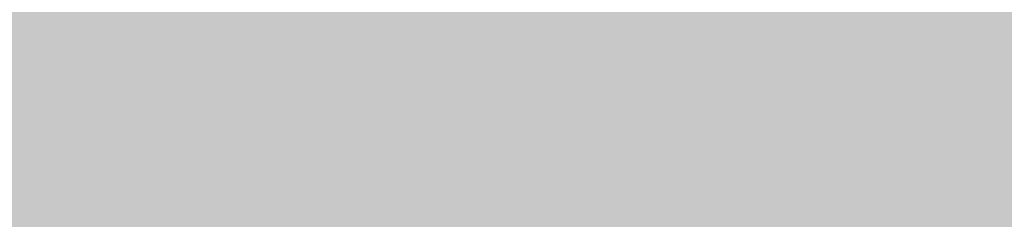
# Model space of a CAD drawing. Units: millimetres. Extents: x 0 to 2267, y 0 to 1823.
# Tile 103 of 256: x 1600.369 to 1605.705, y 1230.439 to 1231.521. Entities that reach past the tile are written whole.
import ezdxf

# ---------------------------------------------------------------- set-up
doc = ezdxf.new("R2010")
doc.units = ezdxf.units.MM
doc.header["$MEASUREMENT"] = 0
doc.layers.add('M-DIMS', color=2, linetype='Continuous', lineweight=25)
doc.layers.add('M-HATC', color=252, linetype='Continuous', lineweight=18)
doc.styles.get("Standard").update_dxf_attribs({"font": 'arial.ttf'})
doc.dimstyles.get("Standard").update_dxf_attribs({"dimtxt": 7, "dimasz": 4, "dimexe": 0.18, "dimexo": 0.0625, "dimgap": 0.09, "dimtad": 0, "dimdec": 0, "dimzin": 0, "dimdsep": 46, "dimtxsty": 'Standard', "dimcen": 0.09, "dimadec": 0, "dimazin": 0, "dimtfac": 1, "dimtdec": 0, "dimtofl": 0, "dimtmove": 0, "dimatfit": 3, "dimfxl": 1, "dimtolj": 1, "dimtzin": 0, "dimarcsym": 0})

# ---------------------------------------------------------------- blocks, each defined once
blk = doc.blocks.new('*D19')
at = {"layer": 'Defpoints', "color": 0, "transparency": 16777216}
for p in [(1605.3399, 1483.3044), (1445.5291, 1333.8851)]:
    blk.add_point(p, dxfattribs=at)
at = {"layer": 'M-DIMS', "color": 0, "lineweight": -2, "transparency": 16777216}
for p, q in [((1605.3399, 1483.2144), (1605.3399, 1483.3944)), ((1605.2499, 1483.3044), (1605.4299, 1483.3044)), ((1366.3244, 1259.8306), (1442.6072, 1331.1532))]:
    blk.add_line(p, q, dxfattribs=at)
at = {"layer": 'M-DIMS', "color": 0, "transparency": 16777216}
blk.add_solid([(1442.1519, 1331.6402), (1443.0625, 1330.6663), (1445.5291, 1333.8851)], dxfattribs=at)
at = {"layer": 'M-DIMS', "color": 0, "transparency": 16777216, "insert": (1349.6425, 1244.2335), "char_height": 7, "attachment_point": 5, "rotation": 43.0753}
blk.add_mtext('\\A1;2X R218.8', dxfattribs=at)

msp = doc.modelspace()

# ---------------------------------------------------------------- hatches: boundary and pattern name
at = {"layer": 'M-HATC'}
h = msp.add_hatch(color=256, dxfattribs=at)
h.dxf.hatch_style = 1
h.paths.add_polyline_path([(2055.771, 1603.062), (1381.0868, 1603.062), (1381.0868, 1598.062), (2055.771, 1598.062)])
h.paths.add_polyline_path([(2055.771, 1598.062), (1381.0868, 1598.062), (1381.0868, 1593.062), (2055.771, 1593.062)])
h.paths.add_polyline_path([(2051.3074, 1536.7609), (1385.5504, 1536.7609), (1385.5504, 1526.7609), (1387.5504, 1526.7609), (1388.5366, 1525.0528), (1385.3319, 1521.2335), (1385.3319, 1521.2226), (2050.2542, 1522.7491), (2048.3212, 1525.0528), (2049.3074, 1526.7609), (2051.3074, 1526.7609)])
edge = h.paths.add_edge_path()
edge.add_arc((1847.5345, 1379.1492), 135, 222.603061, 222.890851, ccw=False)
edge.add_line((1748.1663, 1287.7656), (1683.0921, 1287.7656))
edge.add_arc((1583.7239, 1379.1492), 135, 317.109149, 317.396939, ccw=False)
edge.add_arc((1678.9686, 1290.6707), 5, 222.8909, 317.1091, ccw=False)
edge.add_arc((1774.2133, 1379.1492), 135, 222.603061, 222.890851, ccw=False)
edge.add_line((1674.8451, 1287.7656), (1609.7709, 1287.7656))
edge.add_arc((1510.4027, 1379.1492), 135, 317.109149, 317.396939, ccw=False)
edge.add_arc((1605.6474, 1290.6707), 5, 222.8909, 317.1091, ccw=False)
edge.add_arc((1700.8921, 1379.1492), 135, 222.603061, 222.890851, ccw=False)
edge.add_line((1601.5239, 1287.7656), (1536.4497, 1287.7656))
edge.add_arc((1437.0815, 1379.1492), 135, 317.109149, 317.396939, ccw=False)
edge.add_arc((1532.3262, 1290.6707), 5, 222.8909, 317.1091, ccw=False)
edge.add_arc((1627.5709, 1379.1492), 135, 222.603061, 222.890851, ccw=False)
edge.add_line((1528.2027, 1287.7656), (1505.9289, 1287.7656))
edge.add_spline(control_points=[(1505.9289, 1287.7656), (1504.2622, 1287.7656), (1504.2622, 1282.7656), (1505.9289, 1282.7656)], knot_values=[0, 0, 0, 0, 5, 5, 5, 5], degree=3, periodic=0)
edge.add_line((1505.9289, 1282.7656), (1930.9289, 1282.7656))
edge.add_spline(control_points=[(1930.9289, 1282.7656), (1932.5956, 1282.7656), (1932.5956, 1287.7656), (1930.9289, 1287.7656)], knot_values=[0, 0, 0, 0, 5, 5, 5, 5], degree=3, periodic=0)
edge.add_line((1930.9289, 1287.7656), (1903.0557, 1287.7656))
edge.add_arc((1803.6875, 1379.1492), 135, 317.109149, 317.396939, ccw=False)
edge.add_arc((1898.9322, 1290.6707), 5, 222.8909, 317.1091, ccw=False)
edge.add_arc((1994.1769, 1379.1492), 135, 222.603061, 222.890851, ccw=False)
edge.add_line((1894.8087, 1287.7656), (1829.7345, 1287.7656))
edge.add_arc((1730.3663, 1379.1492), 135, 317.109149, 317.396939, ccw=False)
edge.add_arc((1825.611, 1290.6707), 5, 222.8909, 317.1091, ccw=False)
edge.add_arc((1920.8557, 1379.1492), 135, 222.603061, 222.890851, ccw=False)
edge.add_line((1821.4875, 1287.7656), (1756.4133, 1287.7656))
edge.add_arc((1657.0451, 1379.1492), 135, 317.109149, 317.396939, ccw=False)
edge.add_arc((1752.2898, 1290.6707), 5, 222.8909, 317.1091, ccw=False)
edge = h.paths.add_edge_path()
edge.add_spline(control_points=[(1843.4289, 1227.2475), (1845.0956, 1227.2475), (1845.0956, 1232.2475), (1843.4289, 1232.2475)], knot_values=[0, 0, 0, 0, 5, 5, 5, 5], degree=3, periodic=0)
edge.add_line((1843.4289, 1232.2475), (1593.4289, 1232.2475))
edge.add_spline(control_points=[(1593.4289, 1232.2475), (1591.7622, 1232.2475), (1591.7622, 1227.2475), (1593.4289, 1227.2475)], knot_values=[0, 0, 0, 0, 5, 5, 5, 5], degree=3, periodic=0)
edge.add_line((1593.4289, 1227.2475), (1843.4289, 1227.2475))
h.paths.add_polyline_path([(1905.9289, 1127.4171), (1530.9289, 1127.4171, 0.414214), (1520.9289, 1117.4171), (1530.9289, 1117.4171), (1915.9289, 1117.4171, 0.414214)])
edge = h.paths.add_edge_path()
edge.add_arc((1397.0858, 1498.4078), 12.7299, 90.78215, 190.87871, ccw=False)
edge.add_line((1396.912, 1511.1365), (1428.0097, 1511.3488))
edge.add_line((1428.0097, 1511.3488), (1433.0097, 1511.3488))
edge.add_line((1433.0097, 1511.3488), (1434.439, 1511.3488))
edge.add_arc((1419.474, 1498.0804), 20, 41.561, 74.08211)
edge.add_line((1424.9592, 1517.3135), (1399.9351, 1517.2561))
edge.add_spline(control_points=[(1399.9307, 1517.2561), (1399.884, 1517.2131), (1399.8328, 1517.1689), (1399.7774, 1517.1236)], knot_values=[11.567499, 11.567499, 11.567499, 11.567499, 11.814249, 11.814249, 11.814249, 11.814249], degree=3, periodic=0)
edge.add_spline(control_points=[(1399.6328, 1517.0099), (1399.5831, 1516.9721), (1399.5307, 1516.9338), (1399.4759, 1516.8947)], knot_values=[11.167718, 11.167718, 11.167718, 11.167718, 11.365188, 11.365188, 11.365188, 11.365188], degree=3, periodic=0)
edge.add_spline(control_points=[(1399.3398, 1516.8001), (1399.1514, 1516.6719), (1398.9384, 1516.5377), (1398.704, 1516.3994)], knot_values=[10.376405, 10.376405, 10.376405, 10.376405, 11.00994, 11.00994, 11.00994, 11.00994], degree=3, periodic=0)
edge.add_spline(control_points=[(1398.6572, 1516.3719), (1398.5789, 1516.326), (1398.4983, 1516.2797), (1398.4155, 1516.2331)], knot_values=[10.125175, 10.125175, 10.125175, 10.125175, 10.334406, 10.334406, 10.334406, 10.334406], degree=3, periodic=0)
edge.add_spline(control_points=[(1398.2642, 1516.1487), (1398.196, 1516.1111), (1398.1263, 1516.0732), (1398.0555, 1516.0351)], knot_values=[9.832246, 9.832246, 9.832246, 9.832246, 9.999658, 9.999658, 9.999658, 9.999658], degree=3, periodic=0)
edge.add_spline(control_points=[(1397.9987, 1516.0048), (1397.7312, 1515.8621), (1397.446, 1515.7171), (1397.1466, 1515.5714)], knot_values=[9.161808, 9.161808, 9.161808, 9.161808, 9.787769, 9.787769, 9.787769, 9.787769], degree=3, periodic=0)
edge.add_spline(control_points=[(1397.1466, 1515.5714), (1396.8418, 1515.423), (1396.5222, 1515.274), (1396.1914, 1515.1262)], knot_values=[8.524455, 8.524455, 8.524455, 8.524455, 9.161808, 9.161808, 9.161808, 9.161808], degree=3, periodic=0)
edge.add_spline(control_points=[(1396.0777, 1515.0756), (1395.9854, 1515.0348), (1395.8922, 1514.994), (1395.7983, 1514.9534)], knot_values=[8.275193, 8.275193, 8.275193, 8.275193, 8.451726, 8.451726, 8.451726, 8.451726], degree=3, periodic=0)
edge.add_spline(control_points=[(1395.6018, 1514.8691), (1395.4997, 1514.8257), (1395.3968, 1514.7824), (1395.2932, 1514.7394)], knot_values=[7.962917, 7.962917, 7.962917, 7.962917, 8.152764, 8.152764, 8.152764, 8.152764], degree=3, periodic=0)
edge.add_spline(control_points=[(1395.2116, 1514.7057), (1394.8278, 1514.5475), (1394.4345, 1514.3929), (1394.0364, 1514.2442)], knot_values=[7.21254, 7.21254, 7.21254, 7.21254, 7.913148, 7.913148, 7.913148, 7.913148], degree=3, periodic=0)
edge.add_spline(control_points=[(1394.0364, 1514.2442), (1393.7076, 1514.1214), (1393.3754, 1514.0027), (1393.0427, 1513.8895)], knot_values=[6.633733, 6.633733, 6.633733, 6.633733, 7.21254, 7.21254, 7.21254, 7.21254], degree=3, periodic=0)
edge.add_spline(control_points=[(1392.8214, 1513.815), (1392.7198, 1513.7812), (1392.6181, 1513.7479), (1392.5166, 1513.7152)], knot_values=[6.328796, 6.328796, 6.328796, 6.328796, 6.505493, 6.505493, 6.505493, 6.505493], degree=3, periodic=0)
edge.add_spline(control_points=[(1392.5166, 1513.7152), (1392.3187, 1513.6515), (1392.1212, 1513.59), (1391.9244, 1513.531)], knot_values=[5.984605, 5.984605, 5.984605, 5.984605, 6.328796, 6.328796, 6.328796, 6.328796], degree=3, periodic=0)
edge.add_spline(control_points=[(1391.7915, 1513.4915), (1391.3122, 1513.3501), (1390.8384, 1513.2239), (1390.3784, 1513.1171)], knot_values=[5.066697, 5.066697, 5.066697, 5.066697, 5.907055, 5.907055, 5.907055, 5.907055], degree=3, periodic=0)
edge.add_spline(control_points=[(1390.3784, 1513.1171), (1390.1797, 1513.071), (1389.9836, 1513.0284), (1389.7907, 1512.9899)], knot_values=[4.70367, 4.70367, 4.70367, 4.70367, 5.066695, 5.066695, 5.066695, 5.066695], degree=3, periodic=0)
edge.add_spline(control_points=[(1389.422, 1512.9204), (1389.2459, 1512.8892), (1389.0729, 1512.8617), (1388.9036, 1512.8381)], knot_values=[4.130571, 4.130571, 4.130571, 4.130571, 4.469816, 4.469816, 4.469816, 4.469816], degree=3, periodic=0)
edge.add_spline(control_points=[(1388.9036, 1512.8381), (1388.591, 1512.7946), (1388.2911, 1512.7644), (1388.0071, 1512.7494)], knot_values=[3.504031, 3.504031, 3.504031, 3.504031, 4.130571, 4.130571, 4.130571, 4.130571], degree=3, periodic=0)
edge.add_spline(control_points=[(1387.9356, 1512.7459), (1387.8538, 1512.7423), (1387.7733, 1512.74), (1387.6944, 1512.739)], knot_values=[3.268866, 3.268866, 3.268866, 3.268866, 3.451164, 3.451164, 3.451164, 3.451164], degree=3, periodic=0)
edge.add_spline(control_points=[(1387.3351, 1512.7443), (1387.2076, 1512.7499), (1387.0847, 1512.7597), (1386.967, 1512.7739)], knot_values=[2.670686, 2.670686, 2.670686, 2.670686, 2.984, 2.984, 2.984, 2.984], degree=3, periodic=0)
edge.add_spline(control_points=[(1386.8327, 1512.7922), (1386.8209, 1512.7941), (1386.8092, 1512.7959), (1386.7975, 1512.7979)], knot_values=[2.516981, 2.516981, 2.516981, 2.516981, 2.549528, 2.549528, 2.549528, 2.549528], degree=3, periodic=0)
edge.add_spline(control_points=[(1386.4526, 1512.8735), (1386.4257, 1512.881), (1386.3993, 1512.889), (1386.3733, 1512.8972)], knot_values=[2.095869, 2.095869, 2.095869, 2.095869, 2.17941, 2.17941, 2.17941, 2.17941], degree=3, periodic=0)
edge.add_spline(control_points=[(1386.0691, 1513.0189), (1386.0634, 1513.0217), (1386.0577, 1513.0246), (1386.052, 1513.0275)], knot_values=[1.72453, 1.72453, 1.72453, 1.72453, 1.745933, 1.745933, 1.745933, 1.745933], degree=3, periodic=0)
edge.add_arc((1399.474, 1498.0804), 20, 131.82432, 180)
edge.add_arc((1630.3336, 1505.5484), 250.9708, 181.705176, 236.427975)
edge.add_arc((1605.3399, 1483.3044), 218.7822, 238.660829, 243.34961)
edge.add_arc((1647.0911, 1510.3592), 262.8986, 183.129836, 237.853442, ccw=False)
h.paths.add_polyline_path([(1406.5369, 1391.9644, 0.149382), (1491.5506, 1296.4418, -0.129517)], flags=17)
edge = h.paths.add_edge_path()
edge.add_arc((2037.3838, 1498.0804), 20, 0, 48.26587)
edge.add_spline(control_points=[(2050.6973, 1513.0052), (2050.6512, 1512.9847), (2050.6034, 1512.9655), (2050.5539, 1512.9477)], knot_values=[1.835652, 1.835652, 1.835652, 1.835652, 2.000781, 2.000781, 2.000781, 2.000781], degree=3, periodic=0)
edge.add_spline(control_points=[(2050.4616, 1512.9166), (2050.479, 1512.9221), (2050.4963, 1512.9277), (2050.5133, 1512.9335)], knot_values=[2.045477, 2.045477, 2.045477, 2.045477, 2.101389, 2.101389, 2.101389, 2.101389], degree=3, periodic=0)
edge.add_spline(control_points=[(2050.129, 1512.8342), (2050.1984, 1512.8473), (2050.2657, 1512.8623), (2050.3308, 1512.8792)], knot_values=[2.237629, 2.237629, 2.237629, 2.237629, 2.435841, 2.435841, 2.435841, 2.435841], degree=3, periodic=0)
edge.add_spline(control_points=[(2050.0946, 1512.8278), (2050.1061, 1512.8299), (2050.1176, 1512.832), (2050.129, 1512.8342)], knot_values=[2.435841, 2.435841, 2.435841, 2.435841, 2.468321, 2.468321, 2.468321, 2.468321], degree=3, periodic=0)
edge.add_spline(control_points=[(2049.7843, 1512.7851), (2049.8552, 1512.7922), (2049.9243, 1512.8008), (2049.9917, 1512.8109)], knot_values=[2.563852, 2.563852, 2.563852, 2.563852, 2.748541, 2.748541, 2.748541, 2.748541], degree=3, periodic=0)
edge.add_spline(control_points=[(2049.4052, 1512.7617), (2049.5364, 1512.7653), (2049.6629, 1512.773), (2049.7843, 1512.7851)], knot_values=[2.748541, 2.748541, 2.748541, 2.748541, 3.064882, 3.064882, 3.064882, 3.064882], degree=3, periodic=0)
edge.add_spline(control_points=[(2049.1698, 1512.7597), (2049.2336, 1512.7591), (2049.2965, 1512.7594), (2049.3584, 1512.7606)], knot_values=[3.102309, 3.102309, 3.102309, 3.102309, 3.2503, 3.2503, 3.2503, 3.2503], degree=3, periodic=0)
edge.add_spline(control_points=[(2048.8573, 1512.7691), (2048.9638, 1512.7638), (2049.068, 1512.7606), (2049.1698, 1512.7597)], knot_values=[3.2503, 3.2503, 3.2503, 3.2503, 3.486069, 3.486069, 3.486069, 3.486069], degree=3, periodic=0)
edge.add_spline(control_points=[(2048.6924, 1512.7789), (2048.3729, 1512.8009), (2048.0345, 1512.8411), (2047.6817, 1512.897)], knot_values=[3.606429, 3.606429, 3.606429, 3.606429, 4.2989, 4.2989, 4.2989, 4.2989], degree=3, periodic=0)
edge.add_spline(control_points=[(2047.6817, 1512.897), (2047.5458, 1512.9185), (2047.4077, 1512.9424), (2047.2678, 1512.9685)], knot_values=[4.2989, 4.2989, 4.2989, 4.2989, 4.565769, 4.565769, 4.565769, 4.565769], degree=3, periodic=0)
edge.add_spline(control_points=[(2047.2678, 1512.9685), (2047.1449, 1512.9914), (2047.0207, 1513.016), (2046.8951, 1513.0422)], knot_values=[4.565769, 4.565769, 4.565769, 4.565769, 4.799971, 4.799971, 4.799971, 4.799971], degree=3, periodic=0)
edge.add_spline(control_points=[(2046.8951, 1513.0422), (2046.5286, 1513.1188), (2046.1513, 1513.209), (2045.7676, 1513.3107)], knot_values=[4.799971, 4.799971, 4.799971, 4.799971, 5.483718, 5.483718, 5.483718, 5.483718], degree=3, periodic=0)
edge.add_spline(control_points=[(2045.7676, 1513.3107), (2045.3724, 1513.4154), (2044.9704, 1513.5322), (2044.5662, 1513.6588)], knot_values=[5.483718, 5.483718, 5.483718, 5.483718, 6.187866, 6.187866, 6.187866, 6.187866], degree=3, periodic=0)
edge.add_spline(control_points=[(2044.5662, 1513.6588), (2044.4149, 1513.7061), (2044.2633, 1513.7549), (2044.1116, 1513.8048)], knot_values=[6.187866, 6.187866, 6.187866, 6.187866, 6.451551, 6.451551, 6.451551, 6.451551], degree=3, periodic=0)
edge.add_spline(control_points=[(2044.1116, 1513.8048), (2043.9967, 1513.8427), (2043.8817, 1513.8813), (2043.7668, 1513.9205)], knot_values=[6.451551, 6.451551, 6.451551, 6.451551, 6.651434, 6.651434, 6.651434, 6.651434], degree=3, periodic=0)
edge.add_spline(control_points=[(2043.7668, 1513.9205), (2043.3716, 1514.0554), (2042.9774, 1514.1979), (2042.5886, 1514.3458)], knot_values=[6.651434, 6.651434, 6.651434, 6.651434, 7.338879, 7.338879, 7.338879, 7.338879], degree=3, periodic=0)
edge.add_spline(control_points=[(2042.5886, 1514.3458), (2042.1643, 1514.5071), (2041.7465, 1514.6749), (2041.3409, 1514.846)], knot_values=[7.338879, 7.338879, 7.338879, 7.338879, 8.089209, 8.089209, 8.089209, 8.089209], degree=3, periodic=0)
edge.add_spline(control_points=[(2041.3409, 1514.846), (2041.1028, 1514.9465), (2040.869, 1515.0481), (2040.6405, 1515.1502)], knot_values=[8.089209, 8.089209, 8.089209, 8.089209, 8.529587, 8.529587, 8.529587, 8.529587], degree=3, periodic=0)
edge.add_spline(control_points=[(2040.51, 1515.2089), (2040.0824, 1515.4022), (2039.6747, 1515.5971), (2039.295, 1515.7894)], knot_values=[8.613818, 8.613818, 8.613818, 8.613818, 9.44571, 9.44571, 9.44571, 9.44571], degree=3, periodic=0)
edge.add_spline(control_points=[(2039.295, 1515.7894), (2039.0618, 1515.9075), (2038.8391, 1516.0246), (2038.6288, 1516.1398)], knot_values=[9.44571, 9.44571, 9.44571, 9.44571, 9.956404, 9.956404, 9.956404, 9.956404], degree=3, periodic=0)
edge.add_spline(control_points=[(2038.6288, 1516.1398), (2038.5187, 1516.2001), (2038.4121, 1516.2598), (2038.309, 1516.3189)], knot_values=[9.956404, 9.956404, 9.956404, 9.956404, 10.223542, 10.223542, 10.223542, 10.223542], degree=3, periodic=0)
edge.add_spline(control_points=[(2038.309, 1516.3189), (2038.2138, 1516.3735), (2038.1216, 1516.4276), (2038.0328, 1516.481)], knot_values=[10.223542, 10.223542, 10.223542, 10.223542, 10.47051, 10.47051, 10.47051, 10.47051], degree=3, periodic=0)
edge.add_spline(control_points=[(2038.0328, 1516.481), (2037.7855, 1516.6296), (2037.5639, 1516.773), (2037.3722, 1516.909)], knot_values=[10.47051, 10.47051, 10.47051, 10.47051, 11.15767, 11.15767, 11.15767, 11.15767], degree=3, periodic=0)
edge.add_spline(control_points=[(2037.3722, 1516.909), (2037.2789, 1516.9752), (2037.1927, 1517.0396), (2037.1142, 1517.102)], knot_values=[11.15767, 11.15767, 11.15767, 11.15767, 11.49227, 11.49227, 11.49227, 11.49227], degree=3, periodic=0)
edge.add_spline(control_points=[(2036.8564, 1517.3259), (2036.9148, 1517.2692), (2036.9814, 1517.2103), (2037.0557, 1517.1492)], knot_values=[11.577341, 11.577341, 11.577341, 11.577341, 11.91035, 11.91035, 11.91035, 11.91035], degree=3, periodic=0)
edge.add_spline(control_points=[(2036.8074, 1517.3748), (2036.823, 1517.3587), (2036.8393, 1517.3424), (2036.8564, 1517.3259)], knot_values=[11.91035, 11.91035, 11.91035, 11.91035, 12.007402, 12.007402, 12.007402, 12.007402], degree=3, periodic=0)
edge.add_spline(control_points=[(2036.7017, 1517.494), (2036.7104, 1517.483), (2036.7196, 1517.4719), (2036.7291, 1517.4606)], knot_values=[12.184155, 12.184155, 12.184155, 12.184155, 12.255409, 12.255409, 12.255409, 12.255409], degree=3, periodic=0)
edge.add_spline(control_points=[(2036.6159, 1517.6205), (2036.62, 1517.613), (2036.6243, 1517.6055), (2036.6289, 1517.5979)], knot_values=[12.487913, 12.487913, 12.487913, 12.487913, 12.541035, 12.541035, 12.541035, 12.541035], degree=3, periodic=0)
edge.add_spline(control_points=[(2036.5635, 1517.786), (2036.5637, 1517.7794), (2036.5642, 1517.7726), (2036.565, 1517.7658)], knot_values=[12.911761, 12.911761, 12.911761, 12.911761, 12.968286, 12.968286, 12.968286, 12.968286], degree=3, periodic=0)
edge.add_spline(control_points=[(2036.6166, 1517.9304), (2036.6125, 1517.9259), (2036.6086, 1517.9212), (2036.6049, 1517.9165)], knot_values=[13.382527, 13.382527, 13.382527, 13.382527, 13.433791, 13.433791, 13.433791, 13.433791], degree=3, periodic=0)
edge.add_spline(control_points=[(2036.749, 1518.017), (2036.7361, 1518.0116), (2036.7239, 1518.006), (2036.7124, 1518.0002)], knot_values=[13.726299, 13.726299, 13.726299, 13.726299, 13.809928, 13.809928, 13.809928, 13.809928], degree=3, periodic=0)
edge.add_spline(control_points=[(2036.8604, 1518.0528), (2036.8386, 1518.0474), (2036.8181, 1518.0416), (2036.7988, 1518.0353)], knot_values=[13.910887, 13.910887, 13.910887, 13.910887, 14.02153, 14.02153, 14.02153, 14.02153], degree=3, periodic=0)
edge.add_line((2036.9639, 1518.0804), (2032.3838, 1518.0804))
edge.add_line((2032.3838, 1518.0804), (2027.3838, 1518.0804))
edge.add_line((2027.3838, 1518.0804), (2022.3838, 1518.0804))
edge.add_line((2022.3838, 1518.0804), (2017.3838, 1518.0804))
edge.add_arc((2017.3838, 1498.0804), 20, 90, 138.439)
edge.add_line((2002.4188, 1511.3488), (2003.8481, 1511.3488))
edge.add_line((2003.8481, 1511.3488), (2008.8481, 1511.3488))
edge.add_line((2008.8481, 1511.3488), (2039.772, 1511.1377))
edge.add_arc((2039.772, 1498.4078), 12.7299, -10.87871, 90, ccw=False)
edge.add_arc((1789.7668, 1510.3592), 262.8986, 302.146558, 356.870164, ccw=False)
edge.add_arc((1831.5179, 1483.3044), 218.7822, 296.65039, 301.339171)
edge.add_arc((1806.5242, 1505.5484), 250.9708, 303.572025, 358.294824)
h.paths.add_polyline_path([(2030.321, 1391.9644, -0.129517), (1945.3072, 1296.4418, 0.149382)], flags=17)
edge = h.paths.add_edge_path()
edge.add_spline(control_points=[(2037.2464, 1518.0821), (2037.2898, 1518.081), (2037.3355, 1518.0804), (2037.3838, 1518.0804)], knot_values=[0.000012, 0.000012, 0.000012, 0.000012, 0.144754, 0.144754, 0.144754, 0.144754], degree=3, periodic=0)
edge.add_line((2037.3357, 1518.0804), (2037.0096, 1518.0804))
edge.add_spline(control_points=[(2037.0096, 1518.0804), (2036.9822, 1518.0768), (2036.956, 1518.0727), (2036.9312, 1518.0681)], knot_values=[14.13465, 14.13465, 14.13465, 14.13465, 14.247197, 14.247197, 14.247197, 14.247197], degree=3, periodic=0)
edge.add_spline(control_points=[(2036.9312, 1518.0681), (2036.9276, 1518.0674), (2036.9241, 1518.0667), (2036.9205, 1518.0661)], knot_values=[14.118315, 14.118315, 14.118315, 14.118315, 14.13465, 14.13465, 14.13465, 14.13465], degree=3, periodic=0)
edge.add_spline(control_points=[(2036.9205, 1518.0661), (2036.9118, 1518.0644), (2036.9032, 1518.0626), (2036.8948, 1518.0608)], knot_values=[14.078086, 14.078086, 14.078086, 14.078086, 14.118315, 14.118315, 14.118315, 14.118315], degree=3, periodic=0)
edge.add_spline(control_points=[(2036.8948, 1518.0608), (2036.883, 1518.0583), (2036.8716, 1518.0556), (2036.8604, 1518.0528)], knot_values=[14.02153, 14.02153, 14.02153, 14.02153, 14.078086, 14.078086, 14.078086, 14.078086], degree=3, periodic=0)
edge.add_spline(control_points=[(2036.8604, 1518.0528), (2036.8386, 1518.0474), (2036.8181, 1518.0416), (2036.7988, 1518.0353)], knot_values=[13.910887, 13.910887, 13.910887, 13.910887, 14.02153, 14.02153, 14.02153, 14.02153], degree=3, periodic=0)
edge.add_spline(control_points=[(2036.7988, 1518.0353), (2036.7981, 1518.035), (2036.7974, 1518.0348), (2036.7967, 1518.0346)], knot_values=[13.906906, 13.906906, 13.906906, 13.906906, 13.910887, 13.910887, 13.910887, 13.910887], degree=3, periodic=0)
edge.add_spline(control_points=[(2036.7967, 1518.0346), (2036.7882, 1518.0318), (2036.7799, 1518.0289), (2036.7719, 1518.0259)], knot_values=[13.857826, 13.857826, 13.857826, 13.857826, 13.906906, 13.906906, 13.906906, 13.906906], degree=3, periodic=0)
edge.add_spline(control_points=[(2036.7719, 1518.0259), (2036.764, 1518.023), (2036.7564, 1518.02), (2036.749, 1518.017)], knot_values=[13.809928, 13.809928, 13.809928, 13.809928, 13.857826, 13.857826, 13.857826, 13.857826], degree=3, periodic=0)
edge.add_spline(control_points=[(2036.749, 1518.017), (2036.7361, 1518.0116), (2036.7239, 1518.006), (2036.7124, 1518.0002)], knot_values=[13.726299, 13.726299, 13.726299, 13.726299, 13.809928, 13.809928, 13.809928, 13.809928], degree=3, periodic=0)
edge.add_spline(control_points=[(2036.7124, 1518.0002), (2036.7121, 1518), (2036.7118, 1517.9999), (2036.7115, 1517.9997)], knot_values=[13.723993, 13.723993, 13.723993, 13.723993, 13.726299, 13.726299, 13.726299, 13.726299], degree=3, periodic=0)
edge.add_spline(control_points=[(2036.7115, 1517.9997), (2036.7063, 1517.9971), (2036.7013, 1517.9944), (2036.6965, 1517.9917)], knot_values=[13.686536, 13.686536, 13.686536, 13.686536, 13.723993, 13.723993, 13.723993, 13.723993], degree=3, periodic=0)
edge.add_spline(control_points=[(2036.6965, 1517.9917), (2036.6919, 1517.9891), (2036.6874, 1517.9865), (2036.6831, 1517.9839)], knot_values=[13.651251, 13.651251, 13.651251, 13.651251, 13.686536, 13.686536, 13.686536, 13.686536], degree=3, periodic=0)
edge.add_spline(control_points=[(2036.6831, 1517.9839), (2036.6764, 1517.9798), (2036.67, 1517.9757), (2036.6639, 1517.9714)], knot_values=[13.596804, 13.596804, 13.596804, 13.596804, 13.651251, 13.651251, 13.651251, 13.651251], degree=3, periodic=0)
edge.add_spline(control_points=[(2036.6639, 1517.9714), (2036.6636, 1517.9712), (2036.6633, 1517.9709), (2036.6629, 1517.9707)], knot_values=[13.593956, 13.593956, 13.593956, 13.593956, 13.596804, 13.596804, 13.596804, 13.596804], degree=3, periodic=0)
edge.add_spline(control_points=[(2036.6629, 1517.9707), (2036.6603, 1517.9689), (2036.6577, 1517.967), (2036.6552, 1517.9651)], knot_values=[13.570322, 13.570322, 13.570322, 13.570322, 13.593956, 13.593956, 13.593956, 13.593956], degree=3, periodic=0)
edge.add_spline(control_points=[(2036.6552, 1517.9651), (2036.6525, 1517.9631), (2036.6499, 1517.9611), (2036.6474, 1517.9591)], knot_values=[13.545477, 13.545477, 13.545477, 13.545477, 13.570322, 13.570322, 13.570322, 13.570322], degree=3, periodic=0)
edge.add_spline(control_points=[(2036.6474, 1517.9591), (2036.6472, 1517.9589), (2036.6471, 1517.9588), (2036.6469, 1517.9587)], knot_values=[13.543931, 13.543931, 13.543931, 13.543931, 13.545477, 13.545477, 13.545477, 13.545477], degree=3, periodic=0)
edge.add_spline(control_points=[(2036.6469, 1517.9587), (2036.6412, 1517.9541), (2036.6358, 1517.9494), (2036.6307, 1517.9447)], knot_values=[13.488237, 13.488237, 13.488237, 13.488237, 13.543931, 13.543931, 13.543931, 13.543931], degree=3, periodic=0)
edge.add_spline(control_points=[(2036.6307, 1517.9447), (2036.6282, 1517.9423), (2036.6257, 1517.9399), (2036.6233, 1517.9374)], knot_values=[13.460307, 13.460307, 13.460307, 13.460307, 13.488237, 13.488237, 13.488237, 13.488237], degree=3, periodic=0)
edge.add_spline(control_points=[(2036.6233, 1517.9374), (2036.6215, 1517.9356), (2036.6198, 1517.9338), (2036.6181, 1517.932)], knot_values=[13.439712, 13.439712, 13.439712, 13.439712, 13.460307, 13.460307, 13.460307, 13.460307], degree=3, periodic=0)
edge.add_spline(control_points=[(2036.6181, 1517.932), (2036.6176, 1517.9315), (2036.6171, 1517.9309), (2036.6166, 1517.9304)], knot_values=[13.433791, 13.433791, 13.433791, 13.433791, 13.439712, 13.439712, 13.439712, 13.439712], degree=3, periodic=0)
edge.add_spline(control_points=[(2036.6166, 1517.9304), (2036.6125, 1517.9259), (2036.6086, 1517.9212), (2036.6049, 1517.9165)], knot_values=[13.382527, 13.382527, 13.382527, 13.382527, 13.433791, 13.433791, 13.433791, 13.433791], degree=3, periodic=0)
edge.add_spline(control_points=[(2036.6049, 1517.9165), (2036.6026, 1517.9135), (2036.6004, 1517.9104), (2036.5982, 1517.9074)], knot_values=[13.350017, 13.350017, 13.350017, 13.350017, 13.382527, 13.382527, 13.382527, 13.382527], degree=3, periodic=0)
edge.add_spline(control_points=[(2036.5982, 1517.9074), (2036.5972, 1517.9059), (2036.5962, 1517.9043), (2036.5952, 1517.9028)], knot_values=[13.333922, 13.333922, 13.333922, 13.333922, 13.350017, 13.350017, 13.350017, 13.350017], degree=3, periodic=0)
edge.add_spline(control_points=[(2036.5952, 1517.9028), (2036.5945, 1517.9018), (2036.5939, 1517.9009), (2036.5933, 1517.8999)], knot_values=[13.323828, 13.323828, 13.323828, 13.323828, 13.333922, 13.333922, 13.333922, 13.333922], degree=3, periodic=0)
edge.add_spline(control_points=[(2036.5933, 1517.8999), (2036.5905, 1517.8955), (2036.5879, 1517.8909), (2036.5855, 1517.8864)], knot_values=[13.277545, 13.277545, 13.277545, 13.277545, 13.323828, 13.323828, 13.323828, 13.323828], degree=3, periodic=0)
edge.add_spline(control_points=[(2036.5855, 1517.8864), (2036.5836, 1517.8827), (2036.5817, 1517.8789), (2036.5801, 1517.8751)], knot_values=[13.240119, 13.240119, 13.240119, 13.240119, 13.277545, 13.277545, 13.277545, 13.277545], degree=3, periodic=0)
edge.add_spline(control_points=[(2036.5801, 1517.8751), (2036.5795, 1517.8739), (2036.579, 1517.8727), (2036.5785, 1517.8715)], knot_values=[13.228211, 13.228211, 13.228211, 13.228211, 13.240119, 13.240119, 13.240119, 13.240119], degree=3, periodic=0)
edge.add_spline(control_points=[(2036.5785, 1517.8715), (2036.578, 1517.8702), (2036.5774, 1517.869), (2036.5769, 1517.8677)], knot_values=[13.215717, 13.215717, 13.215717, 13.215717, 13.228211, 13.228211, 13.228211, 13.228211], degree=3, periodic=0)
edge.add_spline(control_points=[(2036.5769, 1517.8677), (2036.5755, 1517.864), (2036.5741, 1517.8603), (2036.5729, 1517.8565)], knot_values=[13.179847, 13.179847, 13.179847, 13.179847, 13.215717, 13.215717, 13.215717, 13.215717], degree=3, periodic=0)
edge.add_spline(control_points=[(2036.5729, 1517.8565), (2036.5713, 1517.8515), (2036.5699, 1517.8464), (2036.5687, 1517.8413)], knot_values=[13.132017, 13.132017, 13.132017, 13.132017, 13.179847, 13.179847, 13.179847, 13.179847], degree=3, periodic=0)
edge.add_spline(control_points=[(2036.5687, 1517.8413), (2036.5684, 1517.8402), (2036.5682, 1517.8392), (2036.568, 1517.8382)], knot_values=[13.122482, 13.122482, 13.122482, 13.122482, 13.132017, 13.132017, 13.132017, 13.132017], degree=3, periodic=0)
edge.add_spline(control_points=[(2036.568, 1517.8382), (2036.5676, 1517.8363), (2036.5672, 1517.8345), (2036.5669, 1517.8327)], knot_values=[13.105592, 13.105592, 13.105592, 13.105592, 13.122482, 13.122482, 13.122482, 13.122482], degree=3, periodic=0)
edge.add_spline(control_points=[(2036.5669, 1517.8327), (2036.5662, 1517.8292), (2036.5657, 1517.8257), (2036.5652, 1517.8222)], knot_values=[13.074063, 13.074063, 13.074063, 13.074063, 13.105592, 13.105592, 13.105592, 13.105592], degree=3, periodic=0)
edge.add_spline(control_points=[(2036.5652, 1517.8222), (2036.5652, 1517.8222), (2036.5652, 1517.8222), (2036.5652, 1517.8222)], knot_values=[13.074043, 13.074043, 13.074043, 13.074043, 13.074063, 13.074063, 13.074063, 13.074063], degree=3, periodic=0)
edge.add_spline(control_points=[(2036.5652, 1517.8222), (2036.5644, 1517.8164), (2036.5639, 1517.8106), (2036.5636, 1517.8046)], knot_values=[13.021884, 13.021884, 13.021884, 13.021884, 13.074043, 13.074043, 13.074043, 13.074043], degree=3, periodic=0)
edge.add_spline(control_points=[(2036.5636, 1517.8046), (2036.5636, 1517.804), (2036.5636, 1517.8034), (2036.5635, 1517.8028)], knot_values=[13.01674, 13.01674, 13.01674, 13.01674, 13.021884, 13.021884, 13.021884, 13.021884], degree=3, periodic=0)
edge.add_spline(control_points=[(2036.5635, 1517.8028), (2036.5634, 1517.8005), (2036.5634, 1517.7982), (2036.5634, 1517.7958)], knot_values=[12.996438, 12.996438, 12.996438, 12.996438, 13.01674, 13.01674, 13.01674, 13.01674], degree=3, periodic=0)
edge.add_spline(control_points=[(2036.5634, 1517.7958), (2036.5633, 1517.7926), (2036.5634, 1517.7893), (2036.5635, 1517.786)], knot_values=[12.968286, 12.968286, 12.968286, 12.968286, 12.996438, 12.996438, 12.996438, 12.996438], degree=3, periodic=0)
edge.add_spline(control_points=[(2036.5635, 1517.786), (2036.5637, 1517.7794), (2036.5642, 1517.7726), (2036.565, 1517.7658)], knot_values=[12.911761, 12.911761, 12.911761, 12.911761, 12.968286, 12.968286, 12.968286, 12.968286], degree=3, periodic=0)
edge.add_spline(control_points=[(2036.565, 1517.7658), (2036.565, 1517.7657), (2036.565, 1517.7656), (2036.565, 1517.7656)], knot_values=[12.911017, 12.911017, 12.911017, 12.911017, 12.911761, 12.911761, 12.911761, 12.911761], degree=3, periodic=0)
edge.add_spline(control_points=[(2036.565, 1517.7656), (2036.5654, 1517.7625), (2036.5658, 1517.7593), (2036.5663, 1517.7562)], knot_values=[12.88528, 12.88528, 12.88528, 12.88528, 12.911017, 12.911017, 12.911017, 12.911017], degree=3, periodic=0)
edge.add_spline(control_points=[(2036.5663, 1517.7562), (2036.5667, 1517.7534), (2036.5672, 1517.7506), (2036.5677, 1517.7478)], knot_values=[12.862519, 12.862519, 12.862519, 12.862519, 12.88528, 12.88528, 12.88528, 12.88528], degree=3, periodic=0)
edge.add_spline(control_points=[(2036.5677, 1517.7478), (2036.5678, 1517.7474), (2036.5679, 1517.7469), (2036.568, 1517.7465)], knot_values=[12.858885, 12.858885, 12.858885, 12.858885, 12.862519, 12.862519, 12.862519, 12.862519], degree=3, periodic=0)
edge.add_spline(control_points=[(2036.568, 1517.7465), (2036.5692, 1517.7399), (2036.5707, 1517.7332), (2036.5724, 1517.7264)], knot_values=[12.8053, 12.8053, 12.8053, 12.8053, 12.858885, 12.858885, 12.858885, 12.858885], degree=3, periodic=0)
edge.add_spline(control_points=[(2036.5724, 1517.7264), (2036.5734, 1517.7226), (2036.5745, 1517.7187), (2036.5756, 1517.7149)], knot_values=[12.775176, 12.775176, 12.775176, 12.775176, 12.8053, 12.8053, 12.8053, 12.8053], degree=3, periodic=0)
edge.add_spline(control_points=[(2036.5756, 1517.7149), (2036.5763, 1517.7125), (2036.577, 1517.7102), (2036.5778, 1517.7078)], knot_values=[12.756759, 12.756759, 12.756759, 12.756759, 12.775176, 12.775176, 12.775176, 12.775176], degree=3, periodic=0)
edge.add_spline(control_points=[(2036.5778, 1517.7078), (2036.5781, 1517.7067), (2036.5784, 1517.7057), (2036.5787, 1517.7047)], knot_values=[12.748742, 12.748742, 12.748742, 12.748742, 12.756759, 12.756759, 12.756759, 12.756759], degree=3, periodic=0)
edge.add_spline(control_points=[(2036.5787, 1517.7047), (2036.5808, 1517.6983), (2036.5831, 1517.6919), (2036.5856, 1517.6854)], knot_values=[12.69959, 12.69959, 12.69959, 12.69959, 12.748742, 12.748742, 12.748742, 12.748742], degree=3, periodic=0)
edge.add_spline(control_points=[(2036.5856, 1517.6854), (2036.5876, 1517.68), (2036.5898, 1517.6746), (2036.5921, 1517.6692)], knot_values=[12.659038, 12.659038, 12.659038, 12.659038, 12.69959, 12.69959, 12.69959, 12.69959], degree=3, periodic=0)
edge.add_spline(control_points=[(2036.5921, 1517.6692), (2036.594, 1517.6648), (2036.5959, 1517.6605), (2036.5979, 1517.6561)], knot_values=[12.626806, 12.626806, 12.626806, 12.626806, 12.659038, 12.659038, 12.659038, 12.659038], degree=3, periodic=0)
edge.add_spline(control_points=[(2036.5979, 1517.6561), (2036.5984, 1517.6551), (2036.5989, 1517.6541), (2036.5993, 1517.6531)], knot_values=[12.619394, 12.619394, 12.619394, 12.619394, 12.626806, 12.626806, 12.626806, 12.626806], degree=3, periodic=0)
edge.add_spline(control_points=[(2036.5993, 1517.6531), (2036.6043, 1517.6424), (2036.6099, 1517.6315), (2036.6159, 1517.6205)], knot_values=[12.541039, 12.541039, 12.541039, 12.541039, 12.619394, 12.619394, 12.619394, 12.619394], degree=3, periodic=0)
edge.add_spline(control_points=[(2036.6159, 1517.6205), (2036.6159, 1517.6205), (2036.6159, 1517.6205), (2036.6159, 1517.6205)], knot_values=[12.541035, 12.541035, 12.541035, 12.541035, 12.541039, 12.541039, 12.541039, 12.541039], degree=3, periodic=0)
edge.add_spline(control_points=[(2036.6159, 1517.6205), (2036.62, 1517.613), (2036.6243, 1517.6055), (2036.6289, 1517.5979)], knot_values=[12.487913, 12.487913, 12.487913, 12.487913, 12.541035, 12.541035, 12.541035, 12.541035], degree=3, periodic=0)
edge.add_spline(control_points=[(2036.6289, 1517.5979), (2036.6326, 1517.5916), (2036.6365, 1517.5853), (2036.6406, 1517.5789)], knot_values=[12.443982, 12.443982, 12.443982, 12.443982, 12.487913, 12.487913, 12.487913, 12.487913], degree=3, periodic=0)
edge.add_spline(control_points=[(2036.6406, 1517.5789), (2036.6414, 1517.5776), (2036.6423, 1517.5763), (2036.6431, 1517.5749)], knot_values=[12.434996, 12.434996, 12.434996, 12.434996, 12.443982, 12.443982, 12.443982, 12.443982], degree=3, periodic=0)
edge.add_spline(control_points=[(2036.6431, 1517.5749), (2036.6531, 1517.5596), (2036.6639, 1517.5439), (2036.6756, 1517.528)], knot_values=[12.329647, 12.329647, 12.329647, 12.329647, 12.434996, 12.434996, 12.434996, 12.434996], degree=3, periodic=0)
edge.add_spline(control_points=[(2036.6756, 1517.528), (2036.6839, 1517.5168), (2036.6925, 1517.5055), (2036.7017, 1517.494)], knot_values=[12.255409, 12.255409, 12.255409, 12.255409, 12.329647, 12.329647, 12.329647, 12.329647], degree=3, periodic=0)
edge.add_spline(control_points=[(2036.7017, 1517.494), (2036.7104, 1517.483), (2036.7196, 1517.4719), (2036.7291, 1517.4606)], knot_values=[12.184155, 12.184155, 12.184155, 12.184155, 12.255409, 12.255409, 12.255409, 12.255409], degree=3, periodic=0)
edge.add_spline(control_points=[(2036.7291, 1517.4606), (2036.7436, 1517.4435), (2036.759, 1517.4262), (2036.7753, 1517.4085)], knot_values=[12.075961, 12.075961, 12.075961, 12.075961, 12.184155, 12.184155, 12.184155, 12.184155], degree=3, periodic=0)
edge.add_spline(control_points=[(2036.7753, 1517.4085), (2036.7763, 1517.4075), (2036.7773, 1517.4064), (2036.7783, 1517.4054)], knot_values=[12.069502, 12.069502, 12.069502, 12.069502, 12.075961, 12.075961, 12.075961, 12.075961], degree=3, periodic=0)
edge.add_spline(control_points=[(2036.7783, 1517.4054), (2036.7877, 1517.3953), (2036.7974, 1517.385), (2036.8074, 1517.3748)], knot_values=[12.007402, 12.007402, 12.007402, 12.007402, 12.069502, 12.069502, 12.069502, 12.069502], degree=3, periodic=0)
edge.add_spline(control_points=[(2036.8074, 1517.3748), (2036.823, 1517.3587), (2036.8393, 1517.3424), (2036.8564, 1517.3259)], knot_values=[11.91035, 11.91035, 11.91035, 11.91035, 12.007402, 12.007402, 12.007402, 12.007402], degree=3, periodic=0)
edge.add_spline(control_points=[(2036.8564, 1517.3259), (2036.9148, 1517.2692), (2036.9814, 1517.2103), (2037.0557, 1517.1492)], knot_values=[11.577341, 11.577341, 11.577341, 11.577341, 11.91035, 11.91035, 11.91035, 11.91035], degree=3, periodic=0)
edge.add_spline(control_points=[(2037.0557, 1517.1492), (2037.0747, 1517.1336), (2037.0942, 1517.1179), (2037.1142, 1517.102)], knot_values=[11.49227, 11.49227, 11.49227, 11.49227, 11.577341, 11.577341, 11.577341, 11.577341], degree=3, periodic=0)
edge.add_spline(control_points=[(2037.1142, 1517.102), (2037.1927, 1517.0396), (2037.2789, 1516.9752), (2037.3722, 1516.909)], knot_values=[11.15767, 11.15767, 11.15767, 11.15767, 11.49227, 11.49227, 11.49227, 11.49227], degree=3, periodic=0)
edge.add_spline(control_points=[(2037.3722, 1516.909), (2037.5639, 1516.773), (2037.7855, 1516.6296), (2038.0328, 1516.481)], knot_values=[10.47051, 10.47051, 10.47051, 10.47051, 11.15767, 11.15767, 11.15767, 11.15767], degree=3, periodic=0)
edge.add_spline(control_points=[(2038.0328, 1516.481), (2038.1216, 1516.4276), (2038.2138, 1516.3735), (2038.309, 1516.3189)], knot_values=[10.223542, 10.223542, 10.223542, 10.223542, 10.47051, 10.47051, 10.47051, 10.47051], degree=3, periodic=0)
edge.add_spline(control_points=[(2038.309, 1516.3189), (2038.4121, 1516.2598), (2038.5187, 1516.2001), (2038.6288, 1516.1398)], knot_values=[9.956404, 9.956404, 9.956404, 9.956404, 10.223542, 10.223542, 10.223542, 10.223542], degree=3, periodic=0)
edge.add_spline(control_points=[(2038.6288, 1516.1398), (2038.8391, 1516.0246), (2039.0618, 1515.9075), (2039.295, 1515.7894)], knot_values=[9.44571, 9.44571, 9.44571, 9.44571, 9.956404, 9.956404, 9.956404, 9.956404], degree=3, periodic=0)
edge.add_spline(control_points=[(2039.295, 1515.7894), (2039.6747, 1515.5971), (2040.0824, 1515.4022), (2040.51, 1515.2089)], knot_values=[8.613818, 8.613818, 8.613818, 8.613818, 9.44571, 9.44571, 9.44571, 9.44571], degree=3, periodic=0)
edge.add_spline(control_points=[(2040.51, 1515.2089), (2040.5533, 1515.1893), (2040.5968, 1515.1697), (2040.6405, 1515.1502)], knot_values=[8.529587, 8.529587, 8.529587, 8.529587, 8.613818, 8.613818, 8.613818, 8.613818], degree=3, periodic=0)
edge.add_spline(control_points=[(2040.6405, 1515.1502), (2040.869, 1515.0481), (2041.1028, 1514.9465), (2041.3409, 1514.846)], knot_values=[8.089209, 8.089209, 8.089209, 8.089209, 8.529587, 8.529587, 8.529587, 8.529587], degree=3, periodic=0)
edge.add_spline(control_points=[(2041.3409, 1514.846), (2041.7465, 1514.6749), (2042.1643, 1514.5071), (2042.5886, 1514.3458)], knot_values=[7.338879, 7.338879, 7.338879, 7.338879, 8.089209, 8.089209, 8.089209, 8.089209], degree=3, periodic=0)
edge.add_spline(control_points=[(2042.5886, 1514.3458), (2042.9774, 1514.1979), (2043.3716, 1514.0554), (2043.7668, 1513.9205)], knot_values=[6.651434, 6.651434, 6.651434, 6.651434, 7.338879, 7.338879, 7.338879, 7.338879], degree=3, periodic=0)
edge.add_spline(control_points=[(2043.7668, 1513.9205), (2043.8817, 1513.8813), (2043.9967, 1513.8427), (2044.1116, 1513.8048)], knot_values=[6.451551, 6.451551, 6.451551, 6.451551, 6.651434, 6.651434, 6.651434, 6.651434], degree=3, periodic=0)
edge.add_spline(control_points=[(2044.1116, 1513.8048), (2044.2633, 1513.7549), (2044.4149, 1513.7061), (2044.5662, 1513.6588)], knot_values=[6.187866, 6.187866, 6.187866, 6.187866, 6.451551, 6.451551, 6.451551, 6.451551], degree=3, periodic=0)
edge.add_spline(control_points=[(2044.5662, 1513.6588), (2044.9704, 1513.5322), (2045.3724, 1513.4154), (2045.7676, 1513.3107)], knot_values=[5.483718, 5.483718, 5.483718, 5.483718, 6.187866, 6.187866, 6.187866, 6.187866], degree=3, periodic=0)
edge.add_spline(control_points=[(2045.7676, 1513.3107), (2046.1513, 1513.209), (2046.5286, 1513.1188), (2046.8951, 1513.0422)], knot_values=[4.799971, 4.799971, 4.799971, 4.799971, 5.483718, 5.483718, 5.483718, 5.483718], degree=3, periodic=0)
edge.add_spline(control_points=[(2046.8951, 1513.0422), (2047.0207, 1513.016), (2047.1449, 1512.9914), (2047.2678, 1512.9685)], knot_values=[4.565769, 4.565769, 4.565769, 4.565769, 4.799971, 4.799971, 4.799971, 4.799971], degree=3, periodic=0)
edge.add_spline(control_points=[(2047.2678, 1512.9685), (2047.4077, 1512.9424), (2047.5458, 1512.9185), (2047.6817, 1512.897)], knot_values=[4.2989, 4.2989, 4.2989, 4.2989, 4.565769, 4.565769, 4.565769, 4.565769], degree=3, periodic=0)
edge.add_spline(control_points=[(2047.6817, 1512.897), (2048.0345, 1512.8411), (2048.3729, 1512.8009), (2048.6924, 1512.7789)], knot_values=[3.606429, 3.606429, 3.606429, 3.606429, 4.2989, 4.2989, 4.2989, 4.2989], degree=3, periodic=0)
edge.add_spline(control_points=[(2048.6924, 1512.7789), (2048.7479, 1512.7751), (2048.8029, 1512.7718), (2048.8573, 1512.7691)], knot_values=[3.486069, 3.486069, 3.486069, 3.486069, 3.606429, 3.606429, 3.606429, 3.606429], degree=3, periodic=0)
edge.add_spline(control_points=[(2048.8573, 1512.7691), (2048.9638, 1512.7638), (2049.068, 1512.7606), (2049.1698, 1512.7597)], knot_values=[3.2503, 3.2503, 3.2503, 3.2503, 3.486069, 3.486069, 3.486069, 3.486069], degree=3, periodic=0)
edge.add_spline(control_points=[(2049.1698, 1512.7597), (2049.2336, 1512.7591), (2049.2965, 1512.7594), (2049.3584, 1512.7606)], knot_values=[3.102309, 3.102309, 3.102309, 3.102309, 3.2503, 3.2503, 3.2503, 3.2503], degree=3, periodic=0)
edge.add_spline(control_points=[(2049.3584, 1512.7606), (2049.3741, 1512.7609), (2049.3897, 1512.7613), (2049.4052, 1512.7617)], knot_values=[3.064882, 3.064882, 3.064882, 3.064882, 3.102309, 3.102309, 3.102309, 3.102309], degree=3, periodic=0)
edge.add_spline(control_points=[(2049.4052, 1512.7617), (2049.5364, 1512.7653), (2049.6629, 1512.773), (2049.7843, 1512.7851)], knot_values=[2.748541, 2.748541, 2.748541, 2.748541, 3.064882, 3.064882, 3.064882, 3.064882], degree=3, periodic=0)
edge.add_spline(control_points=[(2049.7843, 1512.7851), (2049.8552, 1512.7922), (2049.9243, 1512.8008), (2049.9917, 1512.8109)], knot_values=[2.563852, 2.563852, 2.563852, 2.563852, 2.748541, 2.748541, 2.748541, 2.748541], degree=3, periodic=0)
edge.add_spline(control_points=[(2049.9917, 1512.8109), (2050.0265, 1512.8161), (2050.0608, 1512.8218), (2050.0946, 1512.8278)], knot_values=[2.468321, 2.468321, 2.468321, 2.468321, 2.563852, 2.563852, 2.563852, 2.563852], degree=3, periodic=0)
edge.add_spline(control_points=[(2050.0946, 1512.8278), (2050.1061, 1512.8299), (2050.1176, 1512.832), (2050.129, 1512.8342)], knot_values=[2.435841, 2.435841, 2.435841, 2.435841, 2.468321, 2.468321, 2.468321, 2.468321], degree=3, periodic=0)
edge.add_spline(control_points=[(2050.129, 1512.8342), (2050.1984, 1512.8473), (2050.2657, 1512.8623), (2050.3308, 1512.8792)], knot_values=[2.237629, 2.237629, 2.237629, 2.237629, 2.435841, 2.435841, 2.435841, 2.435841], degree=3, periodic=0)
edge.add_spline(control_points=[(2050.3308, 1512.8792), (2050.3754, 1512.8908), (2050.4191, 1512.9032), (2050.4616, 1512.9166)], knot_values=[2.101389, 2.101389, 2.101389, 2.101389, 2.237629, 2.237629, 2.237629, 2.237629], degree=3, periodic=0)
edge.add_spline(control_points=[(2050.4616, 1512.9166), (2050.479, 1512.9221), (2050.4963, 1512.9277), (2050.5133, 1512.9335)], knot_values=[2.045477, 2.045477, 2.045477, 2.045477, 2.101389, 2.101389, 2.101389, 2.101389], degree=3, periodic=0)
edge.add_spline(control_points=[(2050.5133, 1512.9335), (2050.527, 1512.9382), (2050.5405, 1512.9429), (2050.5539, 1512.9477)], knot_values=[2.000781, 2.000781, 2.000781, 2.000781, 2.045477, 2.045477, 2.045477, 2.045477], degree=3, periodic=0)
edge.add_spline(control_points=[(2050.5539, 1512.9477), (2050.6034, 1512.9655), (2050.6512, 1512.9847), (2050.6973, 1513.0052)], knot_values=[1.835652, 1.835652, 1.835652, 1.835652, 2.000781, 2.000781, 2.000781, 2.000781], degree=3, periodic=0)
edge.add_arc((2037.3838, 1498.0804), 20, 48.26587, 90.12993)
edge = h.paths.add_edge_path(flags=16)
edge.add_spline(control_points=[(1386.1389, 1512.9859), (1388.92, 1511.7395), (1398.0387, 1515.5187), (1399.9307, 1517.2561)], knot_values=[1.831046, 1.831046, 1.831046, 1.831046, 11.814249, 11.814249, 11.814249, 11.814249], degree=3, periodic=0)
edge.add_line((1399.9307, 1517.2561), (1393.7435, 1517.2419))
edge.add_arc((1399.474, 1498.0804), 20, 106.6501, 131.8173)

# ---------------------------------------------------------------- dimensions: what is measured, and where the dimension line sits
at = {"layer": 'M-DIMS'}
dim = msp.add_radius_dim(center=(1605.3399, 1483.3044), mpoint=(1445.5291, 1333.8851), text='2X <>', dimstyle='Standard', override={"dimdec": 1, "dimlfac": 1, "dimrnd": 0, "dimzin": 0, "dimdsep": 46, "dimlunit": 2}, dxfattribs=at)
dim.commit()
dim.dimension.update_dxf_attribs({"geometry": '*D19', "text_midpoint": (1349.6425, 1244.2335), "dimtype": 164})

doc.saveas('drawing.dxf')
